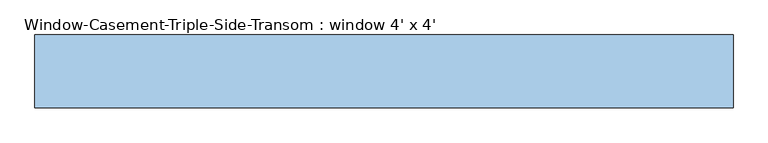
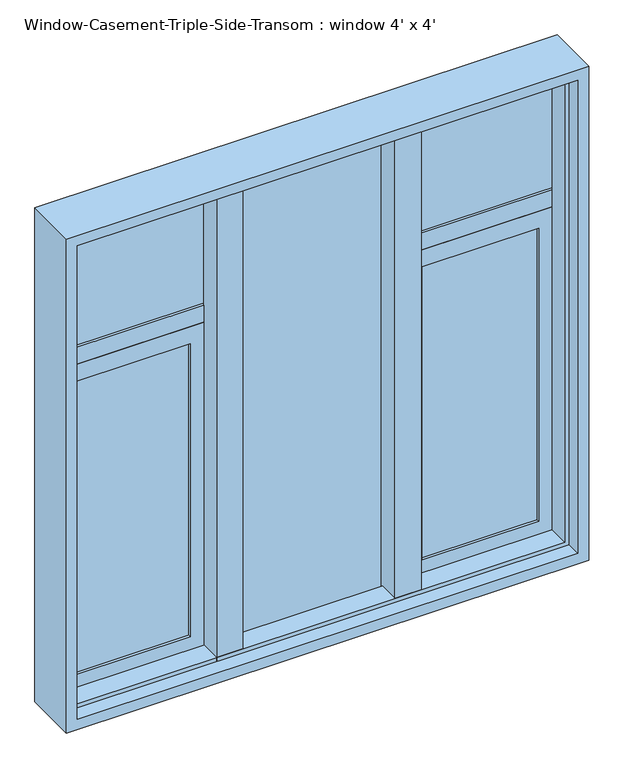
"""IFC4 building model written with IfcOpenShell, lengths in millimetres: window geometry, Window-Casement-Triple-Side-Transom : window 4' x 4'."""

from ifc_helpers import new_model, si_unit, frame, origin, place, context, project, spatial, polyline, outline, extrude, faceted_brep, source, transform, mapped, element, save


def window_casement_triple_side_transom_window_4_x_4_9406f89d(model_context):
    return source(origin(), model_context, "Body", "SolidModel", [
        faceted_brep([(-584.2, 22.225, 2108.2), (-584.2, 63.5, 2108.2), (584.2, 63.5, 2108.2), (584.2, 22.225, 2108.2), (-574.0796875, -28.575, 2098.0796875), (-574.0796875, 22.225, 2098.0796875), (574.0796875, 22.225, 2098.0796875), (574.0796875, -28.575, 2098.0796875), (-584.2, -63.5, 2108.2), (-584.2, -28.575, 2108.2), (584.2, -28.575, 2108.2), (584.2, -63.5, 2108.2), (-609.6, 63.5, 2133.6), (-609.6, -63.5, 2133.6), (609.6, -63.5, 2133.6), (609.6, 63.5, 2133.6), (584.2, 63.5, 939.8), (584.2, 22.225, 939.8), (574.0796875, 22.225, 949.9203125), (574.0796875, -28.575, 949.9203125), (584.2, -28.575, 939.8), (584.2, -63.5, 939.8), (609.6, -63.5, 914.4), (609.6, 63.5, 914.4), (-584.2, 63.5, 939.8), (-584.2, 22.225, 939.8), (-574.0796875, 22.225, 949.9203125), (-574.0796875, -28.575, 949.9203125), (-584.2, -28.575, 939.8), (-584.2, -63.5, 939.8), (-609.6, -63.5, 914.4), (-609.6, 63.5, 914.4)], [[[0, 1, 2, 3]], [[4, 5, 6, 7]], [[8, 9, 10, 11]], [[12, 13, 14, 15]], [[3, 2, 16, 17]], [[7, 6, 18, 19]], [[11, 10, 20, 21]], [[15, 14, 22, 23]], [[17, 16, 24, 25]], [[19, 18, 26, 27]], [[21, 20, 28, 29]], [[23, 22, 30, 31]], [[25, 24, 1, 0]], [[3, 17, 25, 0], [5, 26, 18, 6]], [[27, 26, 5, 4]], [[9, 28, 20, 10], [7, 19, 27, 4]], [[29, 28, 9, 8]], [[13, 30, 22, 14], [11, 21, 29, 8]], [[31, 30, 13, 12]], [[15, 23, 31, 12], [1, 24, 16, 2]]]),
        extrude(outline(polyline([(-177.8, 60.325), (-177.8, -28.575), (-238.7203125, -28.575), (-238.7203125, 22.225), (-228.6, 22.225), (-228.6, 60.325), (-177.8, 60.325)])), frame((0.0, 0.0, 939.8), z_axis=(0.0, 0.0, 1.0), x_axis=(1.0, 0.0, 0.0)), (0.0, 0.0, 1.0), 1168.4),
        extrude(outline(polyline([(228.6, 60.325), (228.6, 22.225), (238.7203125, 22.225), (238.7203125, -28.575), (177.8, -28.575), (177.8, 60.325), (228.6, 60.325)])), frame((0.0, 0.0, 939.8), z_axis=(0.0, 0.0, 1.0), x_axis=(1.0, 0.0, 0.0)), (0.0, 0.0, 1.0), 1168.4),
        extrude(outline(polyline([(1746.9048438, 228.6), (939.8, 228.6), (939.8, 584.2), (1746.9048438, 584.2), (1746.9048438, 228.6)]), holes=[polyline([(1705.0345313, 542.3296875), (981.6703125, 542.3296875), (981.6703125, 270.4703125), (1705.0345313, 270.4703125), (1705.0345313, 542.3296875)])]), frame((0.0, 22.225, 0.0), z_axis=(0.0, 1.0, 0.0), x_axis=(0.0, 0.0, 1.0)), (0.0, 0.0, 1.0), 31.75),
        extrude(outline(polyline([(1746.9048438, -584.2), (939.8, -584.2), (939.8, -228.6), (1746.9048438, -228.6), (1746.9048438, -584.2)]), holes=[polyline([(1705.0345313, -270.4703125), (981.6703125, -270.4703125), (981.6703125, -542.3296875), (1705.0345313, -542.3296875), (1705.0345313, -270.4703125)])]), frame((0.0, 22.225, 0.0), z_axis=(0.0, 1.0, 0.0), x_axis=(0.0, 0.0, 1.0)), (0.0, 0.0, 1.0), 31.75),
        extrude(outline(polyline([(-270.4703125, 47.625), (-270.4703125, 41.275), (-542.3296875, 41.275), (-542.3296875, 47.625), (-270.4703125, 47.625)])), frame((0.0, 0.0, 981.6703125), z_axis=(0.0, 0.0, 1.0), x_axis=(1.0, 0.0, 0.0)), (0.0, 0.0, 1.0), 723.3642188),
        extrude(outline(polyline([(-270.4703125, 34.925), (-270.4703125, 28.575), (-542.3296875, 28.575), (-542.3296875, 34.925), (-270.4703125, 34.925)])), frame((0.0, 0.0, 981.6703125), z_axis=(0.0, 0.0, 1.0), x_axis=(1.0, 0.0, 0.0)), (0.0, 0.0, 1.0), 723.3642188),
        extrude(outline(polyline([(542.3296875, 47.625), (542.3296875, 41.275), (270.4703125, 41.275), (270.4703125, 47.625), (542.3296875, 47.625)])), frame((0.0, 0.0, 981.6703125), z_axis=(0.0, 0.0, 1.0), x_axis=(1.0, 0.0, 0.0)), (0.0, 0.0, 1.0), 723.3642188),
        extrude(outline(polyline([(542.3296875, 34.925), (542.3296875, 28.575), (270.4703125, 28.575), (270.4703125, 34.925), (542.3296875, 34.925)])), frame((0.0, 0.0, 981.6703125), z_axis=(0.0, 0.0, 1.0), x_axis=(1.0, 0.0, 0.0)), (0.0, 0.0, 1.0), 723.3642188),
        extrude(outline(polyline([(584.2, 53.975), (584.2, 22.225), (228.6, 22.225), (228.6, 53.975), (584.2, 53.975)])), frame((0.0, 0.0, 1746.9048438), z_axis=(0.0, 0.0, 1.0), x_axis=(1.0, 0.0, 0.0)), (0.0, 0.0, 1.0), 41.8703125),
        extrude(outline(polyline([(177.8, 47.625), (177.8, 41.275), (-177.8, 41.275), (-177.8, 47.625), (177.8, 47.625)])), frame((0.0, 0.0, 939.8), z_axis=(0.0, 0.0, 1.0), x_axis=(1.0, 0.0, 0.0)), (0.0, 0.0, 1.0), 1168.4),
        extrude(outline(polyline([(177.8, 34.925), (177.8, 28.575), (-177.8, 28.575), (-177.8, 34.925), (177.8, 34.925)])), frame((0.0, 0.0, 939.8), z_axis=(0.0, 0.0, 1.0), x_axis=(1.0, 0.0, 0.0)), (0.0, 0.0, 1.0), 1168.4),
        extrude(outline(polyline([(-228.6, 53.975), (-228.6, 22.225), (-584.2, 22.225), (-584.2, 53.975), (-228.6, 53.975)])), frame((0.0, 0.0, 1746.9048438), z_axis=(0.0, 0.0, 1.0), x_axis=(1.0, 0.0, 0.0)), (0.0, 0.0, 1.0), 41.8703125),
        extrude(outline(polyline([(-228.6, 47.625), (-228.6, 41.275), (-584.2, 41.275), (-584.2, 47.625), (-228.6, 47.625)])), frame((0.0, 0.0, 1788.7751562), z_axis=(0.0, 0.0, 1.0), x_axis=(1.0, 0.0, 0.0)), (0.0, 0.0, 1.0), 319.4248438),
        extrude(outline(polyline([(-228.6, 34.925), (-228.6, 28.575), (-584.2, 28.575), (-584.2, 34.925), (-228.6, 34.925)])), frame((0.0, 0.0, 1788.7751562), z_axis=(0.0, 0.0, 1.0), x_axis=(1.0, 0.0, 0.0)), (0.0, 0.0, 1.0), 319.4248438),
        extrude(outline(polyline([(584.2, 47.625), (584.2, 41.275), (228.6, 41.275), (228.6, 47.625), (584.2, 47.625)])), frame((0.0, 0.0, 1788.7751562), z_axis=(0.0, 0.0, 1.0), x_axis=(1.0, 0.0, 0.0)), (0.0, 0.0, 1.0), 319.4248438),
        extrude(outline(polyline([(584.2, 34.925), (584.2, 28.575), (228.6, 28.575), (228.6, 34.925), (584.2, 34.925)])), frame((0.0, 0.0, 1788.7751562), z_axis=(0.0, 0.0, 1.0), x_axis=(1.0, 0.0, 0.0)), (0.0, 0.0, 1.0), 319.4248438),
    ])


if __name__ == "__main__":
    model = new_model("IFC4")
    model_context = context("Model", 3, world=origin())
    ifc_project = project(units=[si_unit("LENGTHUNIT", "METRE", prefix="MILLI")], contexts=[model_context])
    site = spatial("IfcSite", under=ifc_project)
    building = spatial("IfcBuilding", under=site)
    placement = place(None, origin())
    window_casement_triple_side_transom_window_4_x_4_shape = window_casement_triple_side_transom_window_4_x_4_9406f89d(model_context)
    element("IfcWindow", 1, ObjectType="Window-Casement-Triple-Side-Transom : window 4' x 4'", at=placement, inside=building, context=model_context, shape_type="MappedRepresentation", body=[
        mapped(window_casement_triple_side_transom_window_4_x_4_shape, transform((0.0, 0.0, 0.0), x_axis=(1.0, 0.0, 0.0), y_axis=(0.0, 1.0, 0.0), z_axis=(0.0, 0.0, 1.0))),
    ])
    save(model, "model.ifc")

# Revit data of these elements
# Type "Window-Casement-Triple-Side-Transom : window 4' x 4'"
#   Type Mark = "22"
#   Fire Rating = "0.5h"
#   Assembly Code = "B2020100"
#   Analytic Construction = "Double glazing - domestic"
#   Window Width = 1' - 4"
#   Window Inset [instance default] = 0' - 0 5/8"
#   Wall Thickness [instance default] = 0' - 6"
#   Visual Light Transmittance = 0.81
#   Transom Height Ratio = 0.3
#   Thermal Resistance (R) = 1.8146 (h·ft²·°F)/BTU
#   Solar Heat Gain Coefficient = 0.76
#   Rough Width = 4' - 0 1/2"
#   Rough Height = 4' - 0 1/2"
#   Open Window Height = 2' - 9.6"
#   Heat Transfer Coefficient (U) = 0.5511 BTU/(h·ft²·°F)
#   Height = 4' - 0"
#   Transom Height = 1' - 2.4"
#   Frame Gap 3 [instance default] = 0' - 1 83/128"
#   Frame Gap 2 [instance default] = 0' - 0 5/8"
#   Frame Gap 1 = 0' - 1 51/128"
#   Default Sill Height = 3' - 0"
#   Width = 4' - 0"
#   Frame Material = Metal - Aluminum
#   Glass Panel Material = Glass
#   Wall Closure = (empty or 0)
# Element 1 (IfcWindow, "Window-Casement-Triple-Side-Transom : window 4' x 4'")
#   Wall Thickness = 0' - 5"
#   Materials on its faces: "Metal - Aluminum", "Glass"
# Materials
#   "Metal - Aluminum": class "Metal", colour RGB 247 247 247, transparency 0
#   "Glass": class "Glass", colour RGB 0 128 192, transparency 0.75, Description = "Soda Lime Glass", Cost = 0
